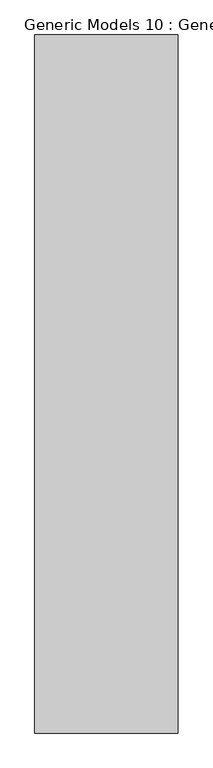
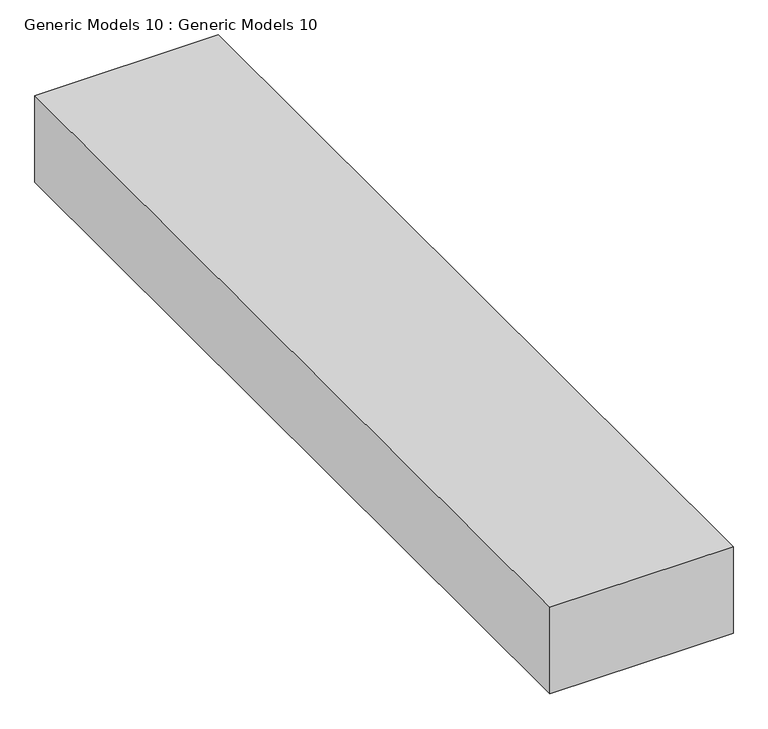
"""IFC4 building model written with IfcOpenShell, lengths in millimetres: proxy geometry, Generic Models 10 : Generic Models 10."""

from ifc_helpers import new_model, si_unit, frame, origin, place, context, project, spatial, polyline, outline, extrude, source, transform, mapped, element, save


def generic_models_10_generic_models_10_ac10314b(model_context):
    return source(origin(), model_context, "Body", "SweptSolid", [
        extrude(outline(polyline([(-14435.0656154, 371.543905), (-14435.0656154, 1855.6844954), (-14130.2656154, 1855.6844954), (-14130.2656154, 371.543905), (-14435.0656154, 371.543905)])), frame((0.0, 0.0, 4948.6955341), z_axis=(0.0, 0.0, 1.0), x_axis=(1.0, 0.0, 0.0)), (0.0, 0.0, 1.0), 152.4),
    ])


if __name__ == "__main__":
    model = new_model("IFC4")
    model_context = context("Model", 3, world=origin())
    ifc_project = project(units=[si_unit("LENGTHUNIT", "METRE", prefix="MILLI")], contexts=[model_context])
    site = spatial("IfcSite", under=ifc_project)
    building = spatial("IfcBuilding", under=site)
    placement = place(None, origin())
    generic_models_10_generic_models_10_shape = generic_models_10_generic_models_10_ac10314b(model_context)
    element("IfcBuildingElementProxy", 1, Name="Generic Models 10 : Generic Models 10", ObjectType="Generic Models 10 : Generic Models 10", at=placement, inside=building, context=model_context, shape_type="MappedRepresentation", body=[
        mapped(generic_models_10_generic_models_10_shape, transform((0.0, 0.0, 0.0), x_axis=(1.0, 0.0, 0.0), y_axis=(0.0, 1.0, 0.0), z_axis=(0.0, 0.0, 1.0))),
    ])
    save(model, "model.ifc")

# Revit data of these elements
# Element 1 (IfcBuildingElementProxy, "Generic Models 10 : Generic Models 10")
#   Materials on its faces: "LIGHT BEIGE"
# Materials
#   "LIGHT BEIGE": class "Generic", colour RGB 120 120 120, transparency 0, Cost = 0
